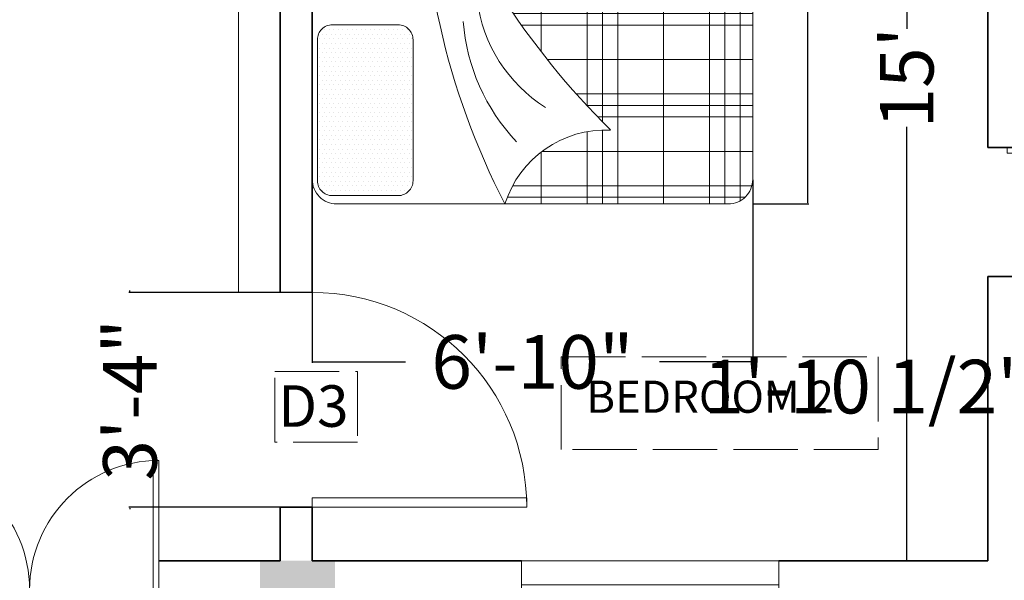
# Model space of a CAD drawing. Units: inches. Extents: x -269 to 4574, y -694 to 313.
# Tile 4 of 19: x 208 to 391, y -360 to -256. Entities that reach past the tile are written whole.
import ezdxf

# ---------------------------------------------------------------- set-up
doc = ezdxf.new("R2010")
doc.units = ezdxf.units.IN
doc.header["$MEASUREMENT"] = 0
doc.linetypes.add('ACAD_ISO02W100', pattern=[15, 12, -3])
for name, color, linetype, lineweight in [('A-ANNO-FRAM', 7, 'ACAD_ISO02W100', 13), ('A-ANNO-IDEN', 6, 'Continuous', 18), ('A-AREA-IDEN', 6, 'Continuous', 20), ('A-COLS', 5, 'Continuous', 35), ('A-FLOR-CASE', 2, 'Continuous', 18), ('A-FURN', 2, 'Continuous', 18), ('DIMENSION', 5, 'Continuous', 18), ('DOORS', 3, 'Continuous', 18), ('WALL', 1, 'Continuous', 35), ('WINDOWS', 2, 'Continuous', 18)]:
    doc.layers.add(name, color=color, linetype=linetype, lineweight=lineweight)
doc.dimstyles.get("Standard").update_dxf_attribs({"dimtxt": 10, "dimasz": 0.18, "dimexe": 0.18, "dimexo": 0.0625, "dimgap": 0.09, "dimtad": 0, "dimdec": 1, "dimzin": 0, "dimdsep": 46, "dimlunit": 3, "dimtxsty": 'Standard', "dimcen": 0.09, "dimclrt": 7, "dimadec": 0, "dimazin": 0, "dimtfac": 1, "dimtdec": 1, "dimtofl": 0, "dimtmove": 0, "dimatfit": 3, "dimfxl": 1, "dimtolj": 1, "dimtzin": 0, "dimarcsym": 0})

# ---------------------------------------------------------------- blocks, each defined once
blk = doc.blocks.new('*U3')
for p, q in [((0, 0), (0, -6)), ((40, 0), (40, -6))]:
    blk.add_line(p, q)
blk.add_lwpolyline([(0, 0), (0, 40), (1.75, 40), (1.75, 0)], close=True)
blk.add_arc((0, 0), 40, 0, 90)
blk = doc.blocks.new('*X12')
at = {"color": 0}
for p, q in [((266.0625, 456.84375), (266.0625, 456.84375)), ((266.25, 456.9375), (266.25, 456.9375)), ((266.25, 456.75), (266.25, 456.75)), ((266.4375, 457.03125), (266.4375, 457.03125)), ((266.4375, 456.84375), (266.4375, 456.84375)), ((266.625, 456.9375), (266.625, 456.9375)), ((266.625, 456.75), (266.625, 456.75)), ((266.8125, 457.03125), (266.8125, 457.03125)), ((266.8125, 456.84375), (266.8125, 456.84375)), ((267, 456.9375), (267, 456.9375)), ((267, 456.75), (267, 456.75)), ((267.1875, 457.03125), (267.1875, 457.03125)), ((267.1875, 456.84375), (267.1875, 456.84375)), ((267.375, 456.9375), (267.375, 456.9375)), ((267.375, 456.75), (267.375, 456.75)), ((267.5625, 457.03125), (267.5625, 457.03125)), ((267.5625, 456.84375), (267.5625, 456.84375)), ((267.75, 456.9375), (267.75, 456.9375)), ((267.75, 456.75), (267.75, 456.75)), ((267.9375, 457.03125), (267.9375, 457.03125)), ((267.9375, 456.84375), (267.9375, 456.84375)), ((268.125, 456.9375), (268.125, 456.9375)), ((268.125, 456.75), (268.125, 456.75)), ((268.3125, 457.03125), (268.3125, 457.03125)), ((268.3125, 456.84375), (268.3125, 456.84375)), ((268.5, 456.9375), (268.5, 456.9375)), ((268.5, 456.75), (268.5, 456.75)), ((268.6875, 457.03125), (268.6875, 457.03125)), ((268.6875, 456.84375), (268.6875, 456.84375)), ((268.875, 456.9375), (268.875, 456.9375)), ((268.875, 456.75), (268.875, 456.75)), ((269.0625, 457.03125), (269.0625, 457.03125)), ((269.0625, 456.84375), (269.0625, 456.84375)), ((269.25, 456.9375), (269.25, 456.9375)), ((269.25, 456.75), (269.25, 456.75)), ((269.4375, 457.03125), (269.4375, 457.03125)), ((269.4375, 456.84375), (269.4375, 456.84375)), ((269.625, 456.9375), (269.625, 456.9375)), ((269.625, 456.75), (269.625, 456.75)), ((269.8125, 457.03125), (269.8125, 457.03125)), ((269.8125, 456.84375), (269.8125, 456.84375)), ((270, 456.9375), (270, 456.9375)), ((270, 456.75), (270, 456.75)), ((270.1875, 457.03125), (270.1875, 457.03125)), ((270.1875, 456.84375), (270.1875, 456.84375)), ((270.375, 456.9375), (270.375, 456.9375)), ((270.375, 456.75), (270.375, 456.75)), ((270.5625, 457.03125), (270.5625, 457.03125)), ((270.5625, 456.84375), (270.5625, 456.84375)), ((270.75, 456.9375), (270.75, 456.9375)), ((270.75, 456.75), (270.75, 456.75)), ((270.9375, 457.03125), (270.9375, 457.03125)), ((270.9375, 456.84375), (270.9375, 456.84375)), ((271.125, 456.9375), (271.125, 456.9375)), ((271.125, 456.75), (271.125, 456.75)), ((271.3125, 457.03125), (271.3125, 457.03125)), ((271.3125, 456.84375), (271.3125, 456.84375)), ((271.5, 456.9375), (271.5, 456.9375)), ((271.5, 456.75), (271.5, 456.75)), ((271.6875, 457.03125), (271.6875, 457.03125)), ((271.6875, 456.84375), (271.6875, 456.84375)), ((271.875, 456.9375), (271.875, 456.9375)), ((271.875, 456.75), (271.875, 456.75)), ((272.0625, 457.03125), (272.0625, 457.03125)), ((272.0625, 456.84375), (272.0625, 456.84375)), ((272.25, 456.9375), (272.25, 456.9375)), ((272.25, 456.75), (272.25, 456.75)), ((272.4375, 456.84375), (272.4375, 456.84375)), ((272.625, 456.75), (272.625, 456.75)), ((265.875, 456.5625), (265.875, 456.5625)), ((265.875, 456.375), (265.875, 456.375)), ((266.0625, 456.65625), (266.0625, 456.65625)), ((266.0625, 456.46875), (266.0625, 456.46875)), ((266.0625, 456.28125), (266.0625, 456.28125)), ((266.25, 456.5625), (266.25, 456.5625)), ((266.25, 456.375), (266.25, 456.375)), ((266.4375, 456.65625), (266.4375, 456.65625)), ((266.4375, 456.46875), (266.4375, 456.46875)), ((266.4375, 456.28125), (266.4375, 456.28125)), ((266.625, 456.5625), (266.625, 456.5625)), ((266.625, 456.375), (266.625, 456.375)), ((266.8125, 456.65625), (266.8125, 456.65625)), ((266.8125, 456.46875), (266.8125, 456.46875)), ((266.8125, 456.28125), (266.8125, 456.28125)), ((267, 456.5625), (267, 456.5625)), ((267, 456.375), (267, 456.375)), ((267.1875, 456.65625), (267.1875, 456.65625)), ((267.1875, 456.46875), (267.1875, 456.46875)), ((267.1875, 456.28125), (267.1875, 456.28125)), ((267.375, 456.5625), (267.375, 456.5625)), ((267.375, 456.375), (267.375, 456.375)), ((267.5625, 456.65625), (267.5625, 456.65625)), ((267.5625, 456.46875), (267.5625, 456.46875)), ((267.5625, 456.28125), (267.5625, 456.28125)), ((267.75, 456.5625), (267.75, 456.5625)), ((267.75, 456.375), (267.75, 456.375)), ((267.9375, 456.65625), (267.9375, 456.65625)), ((267.9375, 456.46875), (267.9375, 456.46875)), ((267.9375, 456.28125), (267.9375, 456.28125)), ((268.125, 456.5625), (268.125, 456.5625)), ((268.125, 456.375), (268.125, 456.375)), ((268.3125, 456.65625), (268.3125, 456.65625)), ((268.3125, 456.46875), (268.3125, 456.46875)), ((268.3125, 456.28125), (268.3125, 456.28125)), ((268.5, 456.5625), (268.5, 456.5625)), ((268.5, 456.375), (268.5, 456.375)), ((268.6875, 456.65625), (268.6875, 456.65625)), ((268.6875, 456.46875), (268.6875, 456.46875)), ((268.6875, 456.28125), (268.6875, 456.28125)), ((268.875, 456.5625), (268.875, 456.5625)), ((268.875, 456.375), (268.875, 456.375)), ((269.0625, 456.65625), (269.0625, 456.65625)), ((269.0625, 456.46875), (269.0625, 456.46875)), ((269.0625, 456.28125), (269.0625, 456.28125)), ((269.25, 456.5625), (269.25, 456.5625)), ((269.25, 456.375), (269.25, 456.375)), ((269.4375, 456.65625), (269.4375, 456.65625)), ((269.4375, 456.46875), (269.4375, 456.46875)), ((269.4375, 456.28125), (269.4375, 456.28125)), ((269.625, 456.5625), (269.625, 456.5625)), ((269.625, 456.375), (269.625, 456.375)), ((269.8125, 456.65625), (269.8125, 456.65625)), ((269.8125, 456.46875), (269.8125, 456.46875)), ((269.8125, 456.28125), (269.8125, 456.28125)), ((270, 456.5625), (270, 456.5625)), ((270, 456.375), (270, 456.375)), ((270.1875, 456.65625), (270.1875, 456.65625)), ((270.1875, 456.46875), (270.1875, 456.46875)), ((270.1875, 456.28125), (270.1875, 456.28125)), ((270.375, 456.5625), (270.375, 456.5625)), ((270.375, 456.375), (270.375, 456.375)), ((270.5625, 456.65625), (270.5625, 456.65625)), ((270.5625, 456.46875), (270.5625, 456.46875)), ((270.5625, 456.28125), (270.5625, 456.28125)), ((270.75, 456.5625), (270.75, 456.5625)), ((270.75, 456.375), (270.75, 456.375)), ((270.9375, 456.65625), (270.9375, 456.65625)), ((270.9375, 456.46875), (270.9375, 456.46875)), ((270.9375, 456.28125), (270.9375, 456.28125)), ((271.125, 456.5625), (271.125, 456.5625)), ((271.125, 456.375), (271.125, 456.375)), ((271.3125, 456.65625), (271.3125, 456.65625)), ((271.3125, 456.46875), (271.3125, 456.46875)), ((271.3125, 456.28125), (271.3125, 456.28125)), ((271.5, 456.5625), (271.5, 456.5625)), ((271.5, 456.375), (271.5, 456.375)), ((271.6875, 456.65625), (271.6875, 456.65625)), ((271.6875, 456.46875), (271.6875, 456.46875)), ((271.6875, 456.28125), (271.6875, 456.28125)), ((271.875, 456.5625), (271.875, 456.5625)), ((271.875, 456.375), (271.875, 456.375)), ((272.0625, 456.65625), (272.0625, 456.65625)), ((272.0625, 456.46875), (272.0625, 456.46875)), ((272.0625, 456.28125), (272.0625, 456.28125)), ((272.25, 456.5625), (272.25, 456.5625)), ((272.25, 456.375), (272.25, 456.375)), ((272.4375, 456.65625), (272.4375, 456.65625)), ((272.4375, 456.46875), (272.4375, 456.46875)), ((272.4375, 456.28125), (272.4375, 456.28125)), ((272.625, 456.5625), (272.625, 456.5625)), ((272.625, 456.375), (272.625, 456.375)), ((272.8125, 456.46875), (272.8125, 456.46875)), ((272.8125, 456.28125), (272.8125, 456.28125)), ((265.875, 456.1875), (265.875, 456.1875)), ((265.875, 456), (265.875, 456)), ((266.0625, 456.09375), (266.0625, 456.09375)), ((266.0625, 455.90625), (266.0625, 455.90625)), ((266.25, 456.1875), (266.25, 456.1875)), ((266.25, 456), (266.25, 456)), ((266.4375, 456.09375), (266.4375, 456.09375)), ((266.4375, 455.90625), (266.4375, 455.90625)), ((266.625, 456.1875), (266.625, 456.1875)), ((266.625, 456), (266.625, 456)), ((266.8125, 456.09375), (266.8125, 456.09375)), ((266.8125, 455.90625), (266.8125, 455.90625)), ((267, 456.1875), (267, 456.1875)), ((267, 456), (267, 456)), ((267.1875, 456.09375), (267.1875, 456.09375)), ((267.1875, 455.90625), (267.1875, 455.90625)), ((267.375, 456.1875), (267.375, 456.1875)), ((267.375, 456), (267.375, 456)), ((267.5625, 456.09375), (267.5625, 456.09375)), ((267.5625, 455.90625), (267.5625, 455.90625)), ((267.75, 456.1875), (267.75, 456.1875)), ((267.75, 456), (267.75, 456)), ((267.9375, 456.09375), (267.9375, 456.09375)), ((267.9375, 455.90625), (267.9375, 455.90625)), ((268.125, 456.1875), (268.125, 456.1875)), ((268.125, 456), (268.125, 456)), ((268.3125, 456.09375), (268.3125, 456.09375)), ((268.3125, 455.90625), (268.3125, 455.90625)), ((268.5, 456.1875), (268.5, 456.1875)), ((268.5, 456), (268.5, 456)), ((268.6875, 456.09375), (268.6875, 456.09375)), ((268.6875, 455.90625), (268.6875, 455.90625)), ((268.875, 456.1875), (268.875, 456.1875)), ((268.875, 456), (268.875, 456)), ((269.0625, 456.09375), (269.0625, 456.09375)), ((269.0625, 455.90625), (269.0625, 455.90625)), ((269.25, 456.1875), (269.25, 456.1875)), ((269.25, 456), (269.25, 456)), ((269.4375, 456.09375), (269.4375, 456.09375)), ((269.4375, 455.90625), (269.4375, 455.90625)), ((269.625, 456.1875), (269.625, 456.1875)), ((269.625, 456), (269.625, 456)), ((269.8125, 456.09375), (269.8125, 456.09375)), ((269.8125, 455.90625), (269.8125, 455.90625)), ((270, 456.1875), (270, 456.1875)), ((270, 456), (270, 456)), ((270.1875, 456.09375), (270.1875, 456.09375)), ((270.1875, 455.90625), (270.1875, 455.90625)), ((270.375, 456.1875), (270.375, 456.1875)), ((270.375, 456), (270.375, 456)), ((270.5625, 456.09375), (270.5625, 456.09375)), ((270.5625, 455.90625), (270.5625, 455.90625)), ((270.75, 456.1875), (270.75, 456.1875)), ((270.75, 456), (270.75, 456)), ((270.9375, 456.09375), (270.9375, 456.09375)), ((270.9375, 455.90625), (270.9375, 455.90625)), ((271.125, 456.1875), (271.125, 456.1875)), ((271.125, 456), (271.125, 456)), ((271.3125, 456.09375), (271.3125, 456.09375)), ((271.3125, 455.90625), (271.3125, 455.90625)), ((271.5, 456.1875), (271.5, 456.1875)), ((271.5, 456), (271.5, 456)), ((271.6875, 456.09375), (271.6875, 456.09375)), ((271.6875, 455.90625), (271.6875, 455.90625)), ((271.875, 456.1875), (271.875, 456.1875)), ((271.875, 456), (271.875, 456)), ((272.0625, 456.09375), (272.0625, 456.09375)), ((272.0625, 455.90625), (272.0625, 455.90625)), ((272.25, 456.1875), (272.25, 456.1875)), ((272.25, 456), (272.25, 456)), ((272.4375, 456.09375), (272.4375, 456.09375)), ((272.4375, 455.90625), (272.4375, 455.90625)), ((272.625, 456.1875), (272.625, 456.1875)), ((272.625, 456), (272.625, 456)), ((272.8125, 456.09375), (272.8125, 456.09375)), ((272.8125, 455.90625), (272.8125, 455.90625)), ((265.875, 455.8125), (265.875, 455.8125)), ((265.875, 455.625), (265.875, 455.625)), ((266.0625, 455.71875), (266.0625, 455.71875)), ((266.0625, 455.53125), (266.0625, 455.53125)), ((266.25, 455.8125), (266.25, 455.8125)), ((266.25, 455.625), (266.25, 455.625)), ((266.4375, 455.71875), (266.4375, 455.71875)), ((266.4375, 455.53125), (266.4375, 455.53125)), ((266.625, 455.8125), (266.625, 455.8125)), ((266.625, 455.625), (266.625, 455.625)), ((266.8125, 455.71875), (266.8125, 455.71875)), ((266.8125, 455.53125), (266.8125, 455.53125)), ((267, 455.8125), (267, 455.8125)), ((267, 455.625), (267, 455.625)), ((267.1875, 455.71875), (267.1875, 455.71875)), ((267.1875, 455.53125), (267.1875, 455.53125)), ((267.375, 455.8125), (267.375, 455.8125)), ((267.375, 455.625), (267.375, 455.625)), ((267.5625, 455.71875), (267.5625, 455.71875)), ((267.5625, 455.53125), (267.5625, 455.53125)), ((267.75, 455.8125), (267.75, 455.8125)), ((267.75, 455.625), (267.75, 455.625)), ((267.9375, 455.71875), (267.9375, 455.71875)), ((267.9375, 455.53125), (267.9375, 455.53125)), ((268.125, 455.8125), (268.125, 455.8125)), ((268.125, 455.625), (268.125, 455.625)), ((268.3125, 455.71875), (268.3125, 455.71875)), ((268.3125, 455.53125), (268.3125, 455.53125)), ((268.5, 455.8125), (268.5, 455.8125)), ((268.5, 455.625), (268.5, 455.625)), ((268.6875, 455.71875), (268.6875, 455.71875)), ((268.6875, 455.53125), (268.6875, 455.53125)), ((268.875, 455.8125), (268.875, 455.8125)), ((268.875, 455.625), (268.875, 455.625)), ((269.0625, 455.71875), (269.0625, 455.71875)), ((269.0625, 455.53125), (269.0625, 455.53125)), ((269.25, 455.8125), (269.25, 455.8125)), ((269.25, 455.625), (269.25, 455.625)), ((269.4375, 455.71875), (269.4375, 455.71875)), ((269.4375, 455.53125), (269.4375, 455.53125)), ((269.625, 455.8125), (269.625, 455.8125)), ((269.625, 455.625), (269.625, 455.625)), ((269.8125, 455.71875), (269.8125, 455.71875)), ((269.8125, 455.53125), (269.8125, 455.53125)), ((270, 455.8125), (270, 455.8125)), ((270, 455.625), (270, 455.625)), ((270.1875, 455.71875), (270.1875, 455.71875)), ((270.1875, 455.53125), (270.1875, 455.53125)), ((270.375, 455.8125), (270.375, 455.8125)), ((270.375, 455.625), (270.375, 455.625)), ((270.5625, 455.71875), (270.5625, 455.71875)), ((270.5625, 455.53125), (270.5625, 455.53125)), ((270.75, 455.8125), (270.75, 455.8125)), ((270.75, 455.625), (270.75, 455.625)), ((270.9375, 455.71875), (270.9375, 455.71875)), ((270.9375, 455.53125), (270.9375, 455.53125)), ((271.125, 455.8125), (271.125, 455.8125)), ((271.125, 455.625), (271.125, 455.625)), ((271.3125, 455.71875), (271.3125, 455.71875)), ((271.3125, 455.53125), (271.3125, 455.53125)), ((271.5, 455.8125), (271.5, 455.8125)), ((271.5, 455.625), (271.5, 455.625)), ((271.6875, 455.71875), (271.6875, 455.71875)), ((271.6875, 455.53125), (271.6875, 455.53125)), ((271.875, 455.8125), (271.875, 455.8125)), ((271.875, 455.625), (271.875, 455.625)), ((272.0625, 455.71875), (272.0625, 455.71875)), ((272.0625, 455.53125), (272.0625, 455.53125)), ((272.25, 455.8125), (272.25, 455.8125)), ((272.25, 455.625), (272.25, 455.625)), ((272.4375, 455.71875), (272.4375, 455.71875)), ((272.4375, 455.53125), (272.4375, 455.53125)), ((272.625, 455.8125), (272.625, 455.8125)), ((272.625, 455.625), (272.625, 455.625)), ((272.8125, 455.71875), (272.8125, 455.71875)), ((272.8125, 455.53125), (272.8125, 455.53125)), ((265.875, 455.4375), (265.875, 455.4375)), ((265.875, 455.25), (265.875, 455.25)), ((266.0625, 455.34375), (266.0625, 455.34375)), ((266.0625, 455.15625), (266.0625, 455.15625)), ((266.25, 455.4375), (266.25, 455.4375)), ((266.25, 455.25), (266.25, 455.25)), ((266.4375, 455.34375), (266.4375, 455.34375)), ((266.4375, 455.15625), (266.4375, 455.15625)), ((266.625, 455.4375), (266.625, 455.4375)), ((266.625, 455.25), (266.625, 455.25)), ((266.8125, 455.34375), (266.8125, 455.34375)), ((266.8125, 455.15625), (266.8125, 455.15625)), ((267, 455.4375), (267, 455.4375)), ((267, 455.25), (267, 455.25)), ((267.1875, 455.34375), (267.1875, 455.34375)), ((267.1875, 455.15625), (267.1875, 455.15625)), ((267.375, 455.4375), (267.375, 455.4375)), ((267.375, 455.25), (267.375, 455.25)), ((267.5625, 455.34375), (267.5625, 455.34375)), ((267.5625, 455.15625), (267.5625, 455.15625)), ((267.75, 455.4375), (267.75, 455.4375)), ((267.75, 455.25), (267.75, 455.25)), ((267.9375, 455.34375), (267.9375, 455.34375)), ((267.9375, 455.15625), (267.9375, 455.15625)), ((268.125, 455.4375), (268.125, 455.4375)), ((268.125, 455.25), (268.125, 455.25)), ((268.3125, 455.34375), (268.3125, 455.34375)), ((268.3125, 455.15625), (268.3125, 455.15625)), ((268.5, 455.4375), (268.5, 455.4375)), ((268.5, 455.25), (268.5, 455.25)), ((268.6875, 455.34375), (268.6875, 455.34375)), ((268.6875, 455.15625), (268.6875, 455.15625)), ((268.875, 455.4375), (268.875, 455.4375)), ((268.875, 455.25), (268.875, 455.25)), ((269.0625, 455.34375), (269.0625, 455.34375)), ((269.0625, 455.15625), (269.0625, 455.15625)), ((269.25, 455.4375), (269.25, 455.4375)), ((269.25, 455.25), (269.25, 455.25)), ((269.4375, 455.34375), (269.4375, 455.34375)), ((269.4375, 455.15625), (269.4375, 455.15625)), ((269.625, 455.4375), (269.625, 455.4375)), ((269.625, 455.25), (269.625, 455.25)), ((269.8125, 455.34375), (269.8125, 455.34375)), ((269.8125, 455.15625), (269.8125, 455.15625)), ((270, 455.4375), (270, 455.4375)), ((270, 455.25), (270, 455.25)), ((270.1875, 455.34375), (270.1875, 455.34375)), ((270.1875, 455.15625), (270.1875, 455.15625)), ((270.375, 455.4375), (270.375, 455.4375)), ((270.375, 455.25), (270.375, 455.25)), ((270.5625, 455.34375), (270.5625, 455.34375)), ((270.5625, 455.15625), (270.5625, 455.15625)), ((270.75, 455.4375), (270.75, 455.4375)), ((270.75, 455.25), (270.75, 455.25)), ((270.9375, 455.34375), (270.9375, 455.34375)), ((270.9375, 455.15625), (270.9375, 455.15625)), ((271.125, 455.4375), (271.125, 455.4375)), ((271.125, 455.25), (271.125, 455.25)), ((271.3125, 455.34375), (271.3125, 455.34375)), ((271.3125, 455.15625), (271.3125, 455.15625)), ((271.5, 455.4375), (271.5, 455.4375)), ((271.5, 455.25), (271.5, 455.25)), ((271.6875, 455.34375), (271.6875, 455.34375)), ((271.6875, 455.15625), (271.6875, 455.15625)), ((271.875, 455.4375), (271.875, 455.4375)), ((271.875, 455.25), (271.875, 455.25)), ((272.0625, 455.34375), (272.0625, 455.34375)), ((272.0625, 455.15625), (272.0625, 455.15625)), ((272.25, 455.4375), (272.25, 455.4375)), ((272.25, 455.25), (272.25, 455.25)), ((272.4375, 455.34375), (272.4375, 455.34375)), ((272.4375, 455.15625), (272.4375, 455.15625)), ((272.625, 455.4375), (272.625, 455.4375)), ((272.625, 455.25), (272.625, 455.25)), ((272.8125, 455.34375), (272.8125, 455.34375)), ((272.8125, 455.15625), (272.8125, 455.15625)), ((265.875, 455.0625), (265.875, 455.0625)), ((265.875, 454.875), (265.875, 454.875)), ((265.875, 454.6875), (265.875, 454.6875)), ((266.0625, 454.96875), (266.0625, 454.96875)), ((266.0625, 454.78125), (266.0625, 454.78125)), ((266.25, 455.0625), (266.25, 455.0625)), ((266.25, 454.875), (266.25, 454.875)), ((266.25, 454.6875), (266.25, 454.6875)), ((266.4375, 454.96875), (266.4375, 454.96875)), ((266.4375, 454.78125), (266.4375, 454.78125)), ((266.625, 455.0625), (266.625, 455.0625)), ((266.625, 454.875), (266.625, 454.875)), ((266.625, 454.6875), (266.625, 454.6875)), ((266.8125, 454.96875), (266.8125, 454.96875)), ((266.8125, 454.78125), (266.8125, 454.78125)), ((267, 455.0625), (267, 455.0625)), ((267, 454.875), (267, 454.875)), ((267, 454.6875), (267, 454.6875)), ((267.1875, 454.96875), (267.1875, 454.96875)), ((267.1875, 454.78125), (267.1875, 454.78125)), ((267.375, 455.0625), (267.375, 455.0625)), ((267.375, 454.875), (267.375, 454.875)), ((267.375, 454.6875), (267.375, 454.6875)), ((267.5625, 454.96875), (267.5625, 454.96875)), ((267.5625, 454.78125), (267.5625, 454.78125)), ((267.75, 455.0625), (267.75, 455.0625)), ((267.75, 454.875), (267.75, 454.875)), ((267.75, 454.6875), (267.75, 454.6875)), ((267.9375, 454.96875), (267.9375, 454.96875)), ((267.9375, 454.78125), (267.9375, 454.78125)), ((268.125, 455.0625), (268.125, 455.0625)), ((268.125, 454.875), (268.125, 454.875)), ((268.125, 454.6875), (268.125, 454.6875)), ((268.3125, 454.96875), (268.3125, 454.96875)), ((268.3125, 454.78125), (268.3125, 454.78125)), ((268.5, 455.0625), (268.5, 455.0625)), ((268.5, 454.875), (268.5, 454.875)), ((268.5, 454.6875), (268.5, 454.6875)), ((268.6875, 454.96875), (268.6875, 454.96875)), ((268.6875, 454.78125), (268.6875, 454.78125)), ((268.875, 455.0625), (268.875, 455.0625)), ((268.875, 454.875), (268.875, 454.875)), ((268.875, 454.6875), (268.875, 454.6875)), ((269.0625, 454.96875), (269.0625, 454.96875)), ((269.0625, 454.78125), (269.0625, 454.78125)), ((269.25, 455.0625), (269.25, 455.0625)), ((269.25, 454.875), (269.25, 454.875)), ((269.25, 454.6875), (269.25, 454.6875)), ((269.4375, 454.96875), (269.4375, 454.96875)), ((269.4375, 454.78125), (269.4375, 454.78125)), ((269.625, 455.0625), (269.625, 455.0625)), ((269.625, 454.875), (269.625, 454.875)), ((269.625, 454.6875), (269.625, 454.6875)), ((269.8125, 454.96875), (269.8125, 454.96875)), ((269.8125, 454.78125), (269.8125, 454.78125)), ((270, 455.0625), (270, 455.0625)), ((270, 454.875), (270, 454.875)), ((270, 454.6875), (270, 454.6875)), ((270.1875, 454.96875), (270.1875, 454.96875)), ((270.1875, 454.78125), (270.1875, 454.78125)), ((270.375, 455.0625), (270.375, 455.0625)), ((270.375, 454.875), (270.375, 454.875)), ((270.375, 454.6875), (270.375, 454.6875)), ((270.5625, 454.96875), (270.5625, 454.96875)), ((270.5625, 454.78125), (270.5625, 454.78125)), ((270.75, 455.0625), (270.75, 455.0625)), ((270.75, 454.875), (270.75, 454.875)), ((270.75, 454.6875), (270.75, 454.6875)), ((270.9375, 454.96875), (270.9375, 454.96875)), ((270.9375, 454.78125), (270.9375, 454.78125)), ((271.125, 455.0625), (271.125, 455.0625)), ((271.125, 454.875), (271.125, 454.875)), ((271.125, 454.6875), (271.125, 454.6875)), ((271.3125, 454.96875), (271.3125, 454.96875)), ((271.3125, 454.78125), (271.3125, 454.78125)), ((271.5, 455.0625), (271.5, 455.0625)), ((271.5, 454.875), (271.5, 454.875)), ((271.5, 454.6875), (271.5, 454.6875)), ((271.6875, 454.96875), (271.6875, 454.96875)), ((271.6875, 454.78125), (271.6875, 454.78125)), ((271.875, 455.0625), (271.875, 455.0625)), ((271.875, 454.875), (271.875, 454.875)), ((271.875, 454.6875), (271.875, 454.6875)), ((272.0625, 454.96875), (272.0625, 454.96875)), ((272.0625, 454.78125), (272.0625, 454.78125)), ((272.25, 455.0625), (272.25, 455.0625)), ((272.25, 454.875), (272.25, 454.875)), ((272.25, 454.6875), (272.25, 454.6875)), ((272.4375, 454.96875), (272.4375, 454.96875)), ((272.4375, 454.78125), (272.4375, 454.78125)), ((272.625, 455.0625), (272.625, 455.0625)), ((272.625, 454.875), (272.625, 454.875)), ((272.625, 454.6875), (272.625, 454.6875)), ((272.8125, 454.96875), (272.8125, 454.96875)), ((272.8125, 454.78125), (272.8125, 454.78125)), ((265.875, 454.5), (265.875, 454.5)), ((265.875, 454.3125), (265.875, 454.3125)), ((266.0625, 454.59375), (266.0625, 454.59375)), ((266.0625, 454.40625), (266.0625, 454.40625)), ((266.25, 454.5), (266.25, 454.5)), ((266.25, 454.3125), (266.25, 454.3125)), ((266.4375, 454.59375), (266.4375, 454.59375)), ((266.4375, 454.40625), (266.4375, 454.40625)), ((266.625, 454.5), (266.625, 454.5)), ((266.625, 454.3125), (266.625, 454.3125)), ((266.8125, 454.59375), (266.8125, 454.59375)), ((266.8125, 454.40625), (266.8125, 454.40625)), ((267, 454.5), (267, 454.5)), ((267, 454.3125), (267, 454.3125)), ((267.1875, 454.59375), (267.1875, 454.59375)), ((267.1875, 454.40625), (267.1875, 454.40625)), ((267.375, 454.5), (267.375, 454.5)), ((267.375, 454.3125), (267.375, 454.3125)), ((267.5625, 454.59375), (267.5625, 454.59375)), ((267.5625, 454.40625), (267.5625, 454.40625)), ((267.75, 454.5), (267.75, 454.5)), ((267.75, 454.3125), (267.75, 454.3125)), ((267.9375, 454.59375), (267.9375, 454.59375)), ((267.9375, 454.40625), (267.9375, 454.40625)), ((268.125, 454.5), (268.125, 454.5)), ((268.125, 454.3125), (268.125, 454.3125)), ((268.3125, 454.59375), (268.3125, 454.59375)), ((268.3125, 454.40625), (268.3125, 454.40625)), ((268.5, 454.5), (268.5, 454.5)), ((268.5, 454.3125), (268.5, 454.3125)), ((268.6875, 454.59375), (268.6875, 454.59375)), ((268.6875, 454.40625), (268.6875, 454.40625)), ((268.875, 454.5), (268.875, 454.5)), ((268.875, 454.3125), (268.875, 454.3125)), ((269.0625, 454.59375), (269.0625, 454.59375)), ((269.0625, 454.40625), (269.0625, 454.40625)), ((269.25, 454.5), (269.25, 454.5)), ((269.25, 454.3125), (269.25, 454.3125)), ((269.4375, 454.59375), (269.4375, 454.59375)), ((269.4375, 454.40625), (269.4375, 454.40625)), ((269.625, 454.5), (269.625, 454.5)), ((269.625, 454.3125), (269.625, 454.3125)), ((269.8125, 454.59375), (269.8125, 454.59375)), ((269.8125, 454.40625), (269.8125, 454.40625)), ((270, 454.5), (270, 454.5)), ((270, 454.3125), (270, 454.3125)), ((270.1875, 454.59375), (270.1875, 454.59375)), ((270.1875, 454.40625), (270.1875, 454.40625)), ((270.375, 454.5), (270.375, 454.5)), ((270.375, 454.3125), (270.375, 454.3125)), ((270.5625, 454.59375), (270.5625, 454.59375)), ((270.5625, 454.40625), (270.5625, 454.40625)), ((270.75, 454.5), (270.75, 454.5)), ((270.75, 454.3125), (270.75, 454.3125)), ((270.9375, 454.59375), (270.9375, 454.59375)), ((270.9375, 454.40625), (270.9375, 454.40625)), ((271.125, 454.5), (271.125, 454.5)), ((271.125, 454.3125), (271.125, 454.3125)), ((271.3125, 454.59375), (271.3125, 454.59375)), ((271.3125, 454.40625), (271.3125, 454.40625)), ((271.5, 454.5), (271.5, 454.5)), ((271.5, 454.3125), (271.5, 454.3125)), ((271.6875, 454.59375), (271.6875, 454.59375)), ((271.6875, 454.40625), (271.6875, 454.40625)), ((271.875, 454.5), (271.875, 454.5)), ((271.875, 454.3125), (271.875, 454.3125)), ((272.0625, 454.59375), (272.0625, 454.59375)), ((272.0625, 454.40625), (272.0625, 454.40625)), ((272.25, 454.5), (272.25, 454.5)), ((272.25, 454.3125), (272.25, 454.3125)), ((272.4375, 454.59375), (272.4375, 454.59375)), ((272.4375, 454.40625), (272.4375, 454.40625)), ((272.625, 454.5), (272.625, 454.5)), ((272.625, 454.3125), (272.625, 454.3125)), ((272.8125, 454.59375), (272.8125, 454.59375)), ((272.8125, 454.40625), (272.8125, 454.40625)), ((265.875, 454.125), (265.875, 454.125)), ((265.875, 453.9375), (265.875, 453.9375)), ((266.0625, 454.21875), (266.0625, 454.21875)), ((266.0625, 454.03125), (266.0625, 454.03125)), ((266.25, 454.125), (266.25, 454.125)), ((266.25, 453.9375), (266.25, 453.9375)), ((266.4375, 454.21875), (266.4375, 454.21875)), ((266.4375, 454.03125), (266.4375, 454.03125)), ((266.625, 454.125), (266.625, 454.125)), ((266.625, 453.9375), (266.625, 453.9375)), ((266.8125, 454.21875), (266.8125, 454.21875)), ((266.8125, 454.03125), (266.8125, 454.03125)), ((267, 454.125), (267, 454.125)), ((267, 453.9375), (267, 453.9375)), ((267.1875, 454.21875), (267.1875, 454.21875)), ((267.1875, 454.03125), (267.1875, 454.03125)), ((267.375, 454.125), (267.375, 454.125)), ((267.375, 453.9375), (267.375, 453.9375)), ((267.5625, 454.21875), (267.5625, 454.21875)), ((267.5625, 454.03125), (267.5625, 454.03125)), ((267.75, 454.125), (267.75, 454.125)), ((267.75, 453.9375), (267.75, 453.9375)), ((267.9375, 454.21875), (267.9375, 454.21875)), ((267.9375, 454.03125), (267.9375, 454.03125)), ((268.125, 454.125), (268.125, 454.125)), ((268.125, 453.9375), (268.125, 453.9375)), ((268.3125, 454.21875), (268.3125, 454.21875)), ((268.3125, 454.03125), (268.3125, 454.03125)), ((268.5, 454.125), (268.5, 454.125)), ((268.5, 453.9375), (268.5, 453.9375)), ((268.6875, 454.21875), (268.6875, 454.21875)), ((268.6875, 454.03125), (268.6875, 454.03125)), ((268.875, 454.125), (268.875, 454.125)), ((268.875, 453.9375), (268.875, 453.9375)), ((269.0625, 454.21875), (269.0625, 454.21875)), ((269.0625, 454.03125), (269.0625, 454.03125)), ((269.25, 454.125), (269.25, 454.125)), ((269.25, 453.9375), (269.25, 453.9375)), ((269.4375, 454.21875), (269.4375, 454.21875)), ((269.4375, 454.03125), (269.4375, 454.03125)), ((269.625, 454.125), (269.625, 454.125)), ((269.625, 453.9375), (269.625, 453.9375)), ((269.8125, 454.21875), (269.8125, 454.21875)), ((269.8125, 454.03125), (269.8125, 454.03125)), ((270, 454.125), (270, 454.125)), ((270, 453.9375), (270, 453.9375)), ((270.1875, 454.21875), (270.1875, 454.21875)), ((270.1875, 454.03125), (270.1875, 454.03125)), ((270.375, 454.125), (270.375, 454.125)), ((270.375, 453.9375), (270.375, 453.9375)), ((270.5625, 454.21875), (270.5625, 454.21875)), ((270.5625, 454.03125), (270.5625, 454.03125)), ((270.75, 454.125), (270.75, 454.125)), ((270.75, 453.9375), (270.75, 453.9375)), ((270.9375, 454.21875), (270.9375, 454.21875)), ((270.9375, 454.03125), (270.9375, 454.03125)), ((271.125, 454.125), (271.125, 454.125)), ((271.125, 453.9375), (271.125, 453.9375)), ((271.3125, 454.21875), (271.3125, 454.21875)), ((271.3125, 454.03125), (271.3125, 454.03125)), ((271.5, 454.125), (271.5, 454.125)), ((271.5, 453.9375), (271.5, 453.9375)), ((271.6875, 454.21875), (271.6875, 454.21875)), ((271.6875, 454.03125), (271.6875, 454.03125)), ((271.875, 454.125), (271.875, 454.125)), ((271.875, 453.9375), (271.875, 453.9375)), ((272.0625, 454.21875), (272.0625, 454.21875)), ((272.0625, 454.03125), (272.0625, 454.03125)), ((272.25, 454.125), (272.25, 454.125)), ((272.25, 453.9375), (272.25, 453.9375)), ((272.4375, 454.21875), (272.4375, 454.21875)), ((272.4375, 454.03125), (272.4375, 454.03125)), ((272.625, 454.125), (272.625, 454.125)), ((272.625, 453.9375), (272.625, 453.9375)), ((272.8125, 454.21875), (272.8125, 454.21875)), ((272.8125, 454.03125), (272.8125, 454.03125)), ((265.875, 453.75), (265.875, 453.75)), ((266.0625, 453.84375), (266.0625, 453.84375)), ((266.0625, 453.65625), (266.0625, 453.65625)), ((266.0625, 453.46875), (266.0625, 453.46875)), ((266.25, 453.75), (266.25, 453.75)), ((266.25, 453.5625), (266.25, 453.5625)), ((266.4375, 453.84375), (266.4375, 453.84375)), ((266.4375, 453.65625), (266.4375, 453.65625)), ((266.4375, 453.46875), (266.4375, 453.46875)), ((266.625, 453.75), (266.625, 453.75)), ((266.625, 453.5625), (266.625, 453.5625)), ((266.8125, 453.84375), (266.8125, 453.84375)), ((266.8125, 453.65625), (266.8125, 453.65625)), ((266.8125, 453.46875), (266.8125, 453.46875)), ((267, 453.75), (267, 453.75)), ((267, 453.5625), (267, 453.5625)), ((267.1875, 453.84375), (267.1875, 453.84375)), ((267.1875, 453.65625), (267.1875, 453.65625)), ((267.1875, 453.46875), (267.1875, 453.46875)), ((267.375, 453.75), (267.375, 453.75)), ((267.375, 453.5625), (267.375, 453.5625)), ((267.5625, 453.84375), (267.5625, 453.84375)), ((267.5625, 453.65625), (267.5625, 453.65625)), ((267.5625, 453.46875), (267.5625, 453.46875)), ((267.75, 453.75), (267.75, 453.75)), ((267.75, 453.5625), (267.75, 453.5625)), ((267.9375, 453.84375), (267.9375, 453.84375)), ((267.9375, 453.65625), (267.9375, 453.65625)), ((267.9375, 453.46875), (267.9375, 453.46875)), ((268.125, 453.75), (268.125, 453.75)), ((268.125, 453.5625), (268.125, 453.5625)), ((268.3125, 453.84375), (268.3125, 453.84375)), ((268.3125, 453.65625), (268.3125, 453.65625)), ((268.3125, 453.46875), (268.3125, 453.46875)), ((268.5, 453.75), (268.5, 453.75)), ((268.5, 453.5625), (268.5, 453.5625)), ((268.6875, 453.84375), (268.6875, 453.84375)), ((268.6875, 453.65625), (268.6875, 453.65625)), ((268.6875, 453.46875), (268.6875, 453.46875)), ((268.875, 453.75), (268.875, 453.75)), ((268.875, 453.5625), (268.875, 453.5625)), ((269.0625, 453.84375), (269.0625, 453.84375)), ((269.0625, 453.65625), (269.0625, 453.65625)), ((269.0625, 453.46875), (269.0625, 453.46875)), ((269.25, 453.75), (269.25, 453.75)), ((269.25, 453.5625), (269.25, 453.5625)), ((269.4375, 453.84375), (269.4375, 453.84375)), ((269.4375, 453.65625), (269.4375, 453.65625)), ((269.4375, 453.46875), (269.4375, 453.46875)), ((269.625, 453.75), (269.625, 453.75)), ((269.625, 453.5625), (269.625, 453.5625)), ((269.8125, 453.84375), (269.8125, 453.84375)), ((269.8125, 453.65625), (269.8125, 453.65625)), ((269.8125, 453.46875), (269.8125, 453.46875)), ((270, 453.75), (270, 453.75)), ((270, 453.5625), (270, 453.5625)), ((270.1875, 453.84375), (270.1875, 453.84375)), ((270.1875, 453.65625), (270.1875, 453.65625)), ((270.1875, 453.46875), (270.1875, 453.46875)), ((270.375, 453.75), (270.375, 453.75)), ((270.375, 453.5625), (270.375, 453.5625)), ((270.5625, 453.84375), (270.5625, 453.84375)), ((270.5625, 453.65625), (270.5625, 453.65625)), ((270.5625, 453.46875), (270.5625, 453.46875)), ((270.75, 453.75), (270.75, 453.75)), ((270.75, 453.5625), (270.75, 453.5625)), ((270.9375, 453.84375), (270.9375, 453.84375)), ((270.9375, 453.65625), (270.9375, 453.65625)), ((270.9375, 453.46875), (270.9375, 453.46875)), ((271.125, 453.75), (271.125, 453.75)), ((271.125, 453.5625), (271.125, 453.5625)), ((271.3125, 453.84375), (271.3125, 453.84375)), ((271.3125, 453.65625), (271.3125, 453.65625)), ((271.3125, 453.46875), (271.3125, 453.46875)), ((271.5, 453.75), (271.5, 453.75)), ((271.5, 453.5625), (271.5, 453.5625)), ((271.6875, 453.84375), (271.6875, 453.84375)), ((271.6875, 453.65625), (271.6875, 453.65625)), ((271.6875, 453.46875), (271.6875, 453.46875)), ((271.875, 453.75), (271.875, 453.75)), ((271.875, 453.5625), (271.875, 453.5625)), ((272.0625, 453.84375), (272.0625, 453.84375)), ((272.0625, 453.65625), (272.0625, 453.65625)), ((272.0625, 453.46875), (272.0625, 453.46875)), ((272.25, 453.75), (272.25, 453.75)), ((272.25, 453.5625), (272.25, 453.5625)), ((272.4375, 453.84375), (272.4375, 453.84375)), ((272.4375, 453.65625), (272.4375, 453.65625)), ((272.4375, 453.46875), (272.4375, 453.46875)), ((272.625, 453.75), (272.625, 453.75)), ((272.625, 453.5625), (272.625, 453.5625)), ((272.8125, 453.84375), (272.8125, 453.84375)), ((272.8125, 453.65625), (272.8125, 453.65625)), ((266.0625, 453.28125), (266.0625, 453.28125)), ((266.25, 453.375), (266.25, 453.375)), ((266.25, 453.1875), (266.25, 453.1875)), ((266.4375, 453.28125), (266.4375, 453.28125)), ((266.625, 453.375), (266.625, 453.375)), ((266.625, 453.1875), (266.625, 453.1875)), ((266.8125, 453.28125), (266.8125, 453.28125)), ((267, 453.375), (267, 453.375)), ((267, 453.1875), (267, 453.1875)), ((267.1875, 453.28125), (267.1875, 453.28125)), ((267.375, 453.375), (267.375, 453.375)), ((267.375, 453.1875), (267.375, 453.1875)), ((267.5625, 453.28125), (267.5625, 453.28125)), ((267.75, 453.375), (267.75, 453.375)), ((267.75, 453.1875), (267.75, 453.1875)), ((267.9375, 453.28125), (267.9375, 453.28125)), ((268.125, 453.375), (268.125, 453.375)), ((268.125, 453.1875), (268.125, 453.1875)), ((268.3125, 453.28125), (268.3125, 453.28125)), ((268.5, 453.375), (268.5, 453.375)), ((268.5, 453.1875), (268.5, 453.1875)), ((268.6875, 453.28125), (268.6875, 453.28125)), ((268.875, 453.375), (268.875, 453.375)), ((268.875, 453.1875), (268.875, 453.1875)), ((269.0625, 453.28125), (269.0625, 453.28125)), ((269.25, 453.375), (269.25, 453.375)), ((269.25, 453.1875), (269.25, 453.1875)), ((269.4375, 453.28125), (269.4375, 453.28125)), ((269.625, 453.375), (269.625, 453.375)), ((269.625, 453.1875), (269.625, 453.1875)), ((269.8125, 453.28125), (269.8125, 453.28125)), ((270, 453.375), (270, 453.375)), ((270, 453.1875), (270, 453.1875)), ((270.1875, 453.28125), (270.1875, 453.28125)), ((270.375, 453.375), (270.375, 453.375)), ((270.375, 453.1875), (270.375, 453.1875)), ((270.5625, 453.28125), (270.5625, 453.28125)), ((270.75, 453.375), (270.75, 453.375)), ((270.75, 453.1875), (270.75, 453.1875)), ((270.9375, 453.28125), (270.9375, 453.28125)), ((271.125, 453.375), (271.125, 453.375)), ((271.125, 453.1875), (271.125, 453.1875)), ((271.3125, 453.28125), (271.3125, 453.28125)), ((271.5, 453.375), (271.5, 453.375)), ((271.5, 453.1875), (271.5, 453.1875)), ((271.6875, 453.28125), (271.6875, 453.28125)), ((271.875, 453.375), (271.875, 453.375)), ((271.875, 453.1875), (271.875, 453.1875)), ((272.0625, 453.28125), (272.0625, 453.28125)), ((272.25, 453.375), (272.25, 453.375)), ((272.25, 453.1875), (272.25, 453.1875)), ((272.4375, 453.28125), (272.4375, 453.28125)), ((272.625, 453.375), (272.625, 453.375))]:
    blk.add_line(p, q, dxfattribs=at)
blk = doc.blocks.new('*D22')
at = {"layer": 'Defpoints', "color": 0, "lineweight": 0, "transparency": 16777216}
for p in [(372.99, -176.73), (388.14, -176.73), (388.14, -356.73)]:
    blk.add_point(p, dxfattribs=at)
at = {"layer": 'DIMENSION', "color": 0, "lineweight": -2, "transparency": 16777216}
for p, q in [((388.07, -176.73), (372.81, -176.73)), ((372.99, -176.91), (372.99, -257.59)), ((372.99, -356.55), (372.99, -275.87)), ((388.07, -356.73), (372.81, -356.73))]:
    blk.add_line(p, q, dxfattribs=at)
at = {"layer": 'DIMENSION', "color": 0, "lineweight": 0, "transparency": 16777216}
for points in [[(372.96, -176.91), (373.02, -176.91), (372.99, -176.73)], [(372.96, -356.55), (373.02, -356.55), (372.99, -356.73)]]:
    blk.add_solid(points, dxfattribs=at)
at = {"layer": 'DIMENSION', "color": 0, "transparency": 16777216, "insert": (372.99, -266.73), "char_height": 10, "attachment_point": 5, "rotation": 90}
blk.add_mtext("\\A1;15'", dxfattribs=at)
blk = doc.blocks.new('GLAZ-48IN')
blk.add_line((4.5, 0), (4.5, 48))
blk.add_lwpolyline([(0, 48), (9, 48), (9, 0), (0, 0)], close=True)
blk = doc.blocks.new('*X10')
at = {"color": 0}
for p, q in [((276.598, 451.25), (280.51, 451.25)), ((275.455, 450.625), (280.51, 450.625)), ((274.411, 450), (280.51, 450)), ((265.51, 448.125), (267.634, 448.125)), ((271.723, 448.125), (280.51, 448.125)), ((265.51, 446.25), (268.465, 446.25)), ((269.519, 446.25), (280.51, 446.25)), ((265.51, 445.625), (268.531, 445.625)), ((268.866, 445.625), (280.51, 445.625)), ((265.51, 445), (280.51, 445)), ((265.51, 443.125), (280.51, 443.125)), ((265.51, 441.25), (280.51, 441.25)), ((265.51, 440.625), (280.51, 440.625)), ((265.634, 440), (280.386, 440))]:
    blk.add_line(p, q, dxfattribs=at)
blk = doc.blocks.new('*X11')
at = {"color": 0}
for p, q in [((280.312, 439.886), (280.312, 452.896)), ((278.906, 439.482), (278.906, 452.338)), ((277.031, 439.482), (277.031, 451.471)), ((277.5, 439.482), (277.5, 451.702)), ((276.562, 439.482), (276.562, 451.231)), ((275.156, 439.482), (275.156, 450.451)), ((265.781, 439.797), (265.781, 449.511)), ((273.75, 439.482), (273.75, 449.576)), ((266.25, 439.517), (266.25, 449.296)), ((273.281, 439.482), (273.281, 449.261)), ((272.812, 439.482), (272.812, 448.934)), ((267.656, 439.482), (267.656, 448.095)), ((271.406, 439.482), (271.406, 447.876)), ((270, 439.482), (270, 446.689)), ((269.531, 439.482), (269.531, 446.262)), ((269.062, 439.482), (269.062, 445.817))]:
    blk.add_line(p, q, dxfattribs=at)
blk = doc.blocks.new('BED-DOUBLE-COVER')
for centre, radius, start, end in [((63.32, -75.96), 137.6, 87.8642, 117.4001), ((118.65, -76.93), 147.29, 109.926, 135.3977), ((36.86, 17.25), 36.85, 94.4436, 133.2788), ((41.52, 23.74), 27.87, 97.2157, 147.6656), ((-5.92, 27.4), 19.71, 357.3792, 72.5379)]:
    blk.add_arc(centre, radius, start, end)
at = {"xscale": 4.5633847399786, "yscale": 4.5633847399786, "zscale": 4.5633847399786}
for name in ['*X11', '*X10']:
    blk.add_blockref(name, (-1211.62, -2005.53), dxfattribs=at)
blk = doc.blocks.new('TAG-DOOR-FRAME')
blk.add_lwpolyline([(0, 13.18), (15.39, 13.18), (15.39, 0), (0, 0)], close=True)
blk = doc.blocks.new('COLUMN-9x14-PLAN')
h = blk.add_hatch(color=256)
h.dxf.hatch_style = 1
h.paths.add_polyline_path([(9, 14), (0, 14), (0, 0), (9, 0), (9, 5)])
blk = doc.blocks.new('*D49')
at = {"layer": 'Defpoints', "color": 0, "lineweight": 0, "transparency": 16777216}
for p in [(344.28, -221.79), (354.55, -221.79), (344.28, -290.24)]:
    blk.add_point(p, dxfattribs=at)
at = {"layer": 'DIMENSION', "color": 0, "lineweight": -2, "transparency": 16777216}
for p, q in [((344.34, -221.79), (354.73, -221.79)), ((354.55, -221.79), (354.55, -221.61)), ((354.55, -290.06), (354.55, -221.97)), ((344.34, -290.24), (354.73, -290.24))]:
    blk.add_line(p, q, dxfattribs=at)
at = {"layer": 'DIMENSION', "color": 0, "lineweight": 0, "transparency": 16777216}
for points in [[(354.52, -221.97), (354.58, -221.97), (354.55, -221.79)], [(354.52, -290.06), (354.58, -290.06), (354.55, -290.24)]]:
    blk.add_solid(points, dxfattribs=at)
at = {"layer": 'DIMENSION', "color": 7, "transparency": 16777216, "insert": (354.55, -133.67), "char_height": 10, "attachment_point": 5, "rotation": 90}
blk.add_mtext('\\A1;COVER 5\'-8 1/2" TYP.', dxfattribs=at)
blk = doc.blocks.new('*D57')
at = {"layer": 'Defpoints', "color": 0, "lineweight": 0, "transparency": 16777216}
for p in [(406.93, -328.51), (402.7, -356.73), (406.93, -356.73)]:
    blk.add_point(p, dxfattribs=at)
at = {"layer": 'DIMENSION', "color": 0, "lineweight": -2, "transparency": 16777216}
for p, q in [((406.87, -328.51), (402.52, -328.51)), ((402.7, -328.69), (402.7, -356.55)), ((406.87, -356.73), (402.52, -356.73)), ((402.7, -356.73), (402.7, -356.91))]:
    blk.add_line(p, q, dxfattribs=at)
at = {"layer": 'DIMENSION', "color": 0, "lineweight": 0, "transparency": 16777216}
for points in [[(402.67, -328.69), (402.73, -328.69), (402.7, -328.51)], [(402.67, -356.55), (402.73, -356.55), (402.7, -356.73)]]:
    blk.add_solid(points, dxfattribs=at)
at = {"layer": 'DIMENSION', "color": 7, "transparency": 16777216, "insert": (402.7, -392), "char_height": 10, "attachment_point": 5, "rotation": 90}
blk.add_mtext('\\A1;WC 2\'-4"', dxfattribs=at)
blk = doc.blocks.new('*D58')
at = {"layer": 'Defpoints', "color": 0, "lineweight": 0, "transparency": 16777216}
for p in [(406.93, -324.28), (406.93, -328.51), (429.34, -328.51)]:
    blk.add_point(p, dxfattribs=at)
at = {"layer": 'DIMENSION', "color": 0, "lineweight": -2, "transparency": 16777216}
for p, q in [((406.93, -324.28), (406.75, -324.28)), ((406.93, -328.45), (406.93, -324.1)), ((429.16, -324.28), (407.11, -324.28)), ((429.34, -328.45), (429.34, -324.1))]:
    blk.add_line(p, q, dxfattribs=at)
at = {"layer": 'DIMENSION', "color": 0, "lineweight": 0, "transparency": 16777216}
for points in [[(407.11, -324.25), (407.11, -324.31), (406.93, -324.28)], [(429.16, -324.25), (429.16, -324.31), (429.34, -324.28)]]:
    blk.add_solid(points, dxfattribs=at)
at = {"layer": 'DIMENSION', "color": 7, "transparency": 16777216, "insert": (365.71, -324.28), "char_height": 10, "attachment_point": 5}
blk.add_mtext('\\A1;1\'-10 1/2"', dxfattribs=at)
blk = doc.blocks.new('*D82')
at = {"layer": 'Defpoints', "color": 0, "lineweight": 0, "transparency": 16777216}
for p in [(262.14, -285.68), (344.28, -285.68), (262.14, -319.68)]:
    blk.add_point(p, dxfattribs=at)
at = {"layer": 'DIMENSION', "color": 0, "lineweight": -2, "transparency": 16777216}
for p, q in [((262.14, -285.74), (262.14, -319.86)), ((344.28, -285.74), (344.28, -319.86)), ((262.32, -319.68), (279.55, -319.68)), ((344.1, -319.68), (326.87, -319.68))]:
    blk.add_line(p, q, dxfattribs=at)
at = {"layer": 'DIMENSION', "color": 0, "lineweight": 0, "transparency": 16777216}
for points in [[(262.32, -319.65), (262.32, -319.71), (262.14, -319.68)], [(344.1, -319.65), (344.1, -319.71), (344.28, -319.68)]]:
    blk.add_solid(points, dxfattribs=at)
at = {"layer": 'DIMENSION', "color": 7, "transparency": 16777216, "insert": (303.21, -319.68), "char_height": 10, "attachment_point": 5}
blk.add_mtext('\\A1;6\'-10"', dxfattribs=at)
blk = doc.blocks.new('*D86')
at = {"layer": 'Defpoints', "color": 0, "lineweight": 0, "transparency": 16777216}
for p in [(228.136997, -306.731691), (262.136997, -306.731691), (262.136997, -346.731691)]:
    blk.add_point(p, dxfattribs=at)
at = {"layer": 'DIMENSION', "color": 0, "lineweight": -2, "transparency": 16777216}
for p, q in [((228.136997, -306.551691), (228.136997, -306.371691)), ((262.074497, -306.731691), (227.956997, -306.731691)), ((262.074497, -346.731691), (227.956997, -346.731691)), ((228.136997, -346.911691), (228.136997, -347.091691))]:
    blk.add_line(p, q, dxfattribs=at)
at = {"layer": 'DIMENSION', "color": 0, "lineweight": 0, "transparency": 16777216}
for points in [[(228.106997, -306.551691), (228.166997, -306.551691), (228.136997, -306.731691)], [(228.106997, -346.911691), (228.166997, -346.911691), (228.136997, -346.731691)]]:
    blk.add_solid(points, dxfattribs=at)
at = {"layer": 'DIMENSION', "color": 7, "transparency": 16777216, "insert": (228.136997, -326.731691), "char_height": 10, "attachment_point": 5, "rotation": 90}
blk.add_mtext('\\A1;3\'-4"', dxfattribs=at)

msp = doc.modelspace()

# ---------------------------------------------------------------- linework, layer by layer
at = {"layer": 'A-ANNO-FRAM'}
msp.add_lwpolyline([(308.58, -318.75), (367.68, -318.75), (367.68, -335.98), (308.58, -335.98)], close=True, dxfattribs=at)
at = {"layer": 'A-FLOR-CASE'}
for p in [(248.41, -176.73), (256.14, -306.73)]:
    msp.add_line(p, (248.41, -306.73), dxfattribs=at)
at = {"layer": 'A-FURN'}
for points in [[(344.28, -226.36), (344.28, -285.68, -0.414214), (339.71, -290.24), (266.7, -290.24, -0.414214), (262.14, -285.68), (262.14, -226.36, -0.414214), (266.7, -221.79), (339.71, -221.79, -0.414214)], [(280.93, -259.63), (280.93, -285.92, -0.414214), (278.15, -288.69), (265.88, -288.69, -0.414214), (263.1, -285.92), (263.1, -259.63, -0.414214), (265.88, -256.86), (278.15, -256.86, -0.414214)]]:
    msp.add_lwpolyline(points, format="xyb", close=True, dxfattribs=at)
at = {"layer": 'WALL'}
for p, q in [((256.14, -306.73), (256.14, -162.44)), ((262.14, -306.73), (262.14, -176.73)), ((388.14, -176.73), (388.14, -279.73)), ((388.14, -279.73), (394.14, -279.73)), ((388.14, -303.73), (394.14, -303.73)), ((388.14, -303.73), (388.14, -356.73)), ((256.14, -356.73), (256.14, -346.73)), ((262.14, -346.73), (256.14, -346.73)), ((262.14, -356.73), (262.14, -346.73)), ((256.14, -356.73), (233.52, -356.73)), ((301.14, -356.73), (262.14, -356.73)), ((388.14, -356.73), (349.14, -356.73))]:
    msp.add_line(p, q, dxfattribs=at)

# ---------------------------------------------------------------- block references
at = {"layer": 'A-ANNO-FRAM'}
msp.add_blockref('TAG-DOOR-FRAME', (255.19, -334.65), dxfattribs=at)
at = {"layer": 'A-COLS', "rotation": 90.0000000000004}
msp.add_blockref('COLUMN-9x14-PLAN', (266.41, -365.72), dxfattribs=at)
at = {"layer": 'A-FURN', "rotation": 90.00000000000024}
msp.add_blockref('BED-DOUBLE-COVER', (344.28, -290.24), dxfattribs=at)
at = {"layer": 'A-FURN', "xscale": 4.5633847399786, "yscale": 4.5633847399786, "zscale": 4.5633847399786, "rotation": 90}
msp.add_blockref('*X12', (2348.75, -1501.87), dxfattribs=at)
at = {"layer": 'DOORS', "xscale": 0.600602616892385, "yscale": 0.600602616892385, "zscale": 0.600602616892385, "rotation": 270}
msp.add_blockref('*U3', (391.74, -279.73), dxfattribs=at)
at = {"layer": 'DOORS', "xscale": -1, "rotation": 270}
msp.add_blockref('*U3', (262.14, -346.73), dxfattribs=at)
at = {"layer": 'DOORS', "yscale": 0.6022719637681349, "zscale": 0.6022719637681349}
for p, xscale in [((185.34, -362.13), 0.6022719637681349), ((233.52, -362.13), -0.6022719637681349)]:
    msp.add_blockref('*U3', p, dxfattribs=dict(at, xscale=xscale))
at = {"layer": 'WINDOWS', "extrusion": (0, 0, -1), "zscale": -1, "rotation": 269.9999999999998}
msp.add_blockref('GLAZ-48IN', (-349.14, -356.73), dxfattribs=at)

# ---------------------------------------------------------------- texts
at = {"layer": 'A-ANNO-IDEN'}
msp.add_text('D3', height=7.741, dxfattribs=at).set_placement((255.78, -331.77))
at = {"layer": 'A-AREA-IDEN'}
msp.add_text('BEDROOM 2 ', height=5.994, dxfattribs=at).set_placement((313.24, -329.16))

# ---------------------------------------------------------------- dimensions: what is measured, and where the dimension line sits
at = {"layer": 'DIMENSION'}
for base, p1, p2, angle, text, picture, middle in [((354.5455, -221.7935), (344.2779, -290.2443), (344.2779, -221.7935), 90, 'COVER <> TYP.', '*D49', (354.5455, -133.6663)), ((402.7, -356.73), (406.93, -328.51), (406.93, -356.73), 270, 'WC <>', '*D57', (402.7, -392))]:
    dim = msp.add_linear_dim(base=base, p1=p1, p2=p2, angle=angle, text=text, dimstyle='Standard', override={"dimdec": 1, "dimlfac": 1, "dimrnd": 0, "dimzin": 1, "dimdsep": 46, "dimlunit": 4, "dimfrac": 2}, dxfattribs=at)
    dim.commit()
    dim.dimension.update_dxf_attribs({"geometry": picture, "text_midpoint": middle})
for base, p1, p2, angle, override, picture, middle in [((372.99, -176.73), (388.14, -356.73), (388.14, -176.73), 90, {"dimclrd": 0, "dimclre": 0, "dimclrt": 0}, '*D22', (372.99, -266.73)), ((262.14, -319.68), (344.28, -285.68), (262.14, -285.68), 180, {"dimdec": 1, "dimlfac": 1, "dimrnd": 0, "dimzin": 1, "dimdsep": 46, "dimlunit": 4, "dimfrac": 2}, '*D82', (303.21, -319.68)), ((228.14, -306.73), (262.14, -346.73), (262.14, -306.73), 90, {"dimdec": 1, "dimlfac": 1, "dimrnd": 0, "dimzin": 1, "dimdsep": 46, "dimlunit": 4, "dimfrac": 2}, '*D86', (228.14, -326.73)), ((406.93, -324.28), (429.34, -328.51), (406.93, -328.51), 180, {"dimdec": 1, "dimlfac": 1, "dimrnd": 0, "dimzin": 1, "dimdsep": 46, "dimlunit": 4, "dimfrac": 2}, '*D58', (365.71, -324.28))]:
    dim = msp.add_linear_dim(base=base, p1=p1, p2=p2, angle=angle, dimstyle='Standard', override=override, dxfattribs=at)
    dim.commit()
    dim.dimension.update_dxf_attribs({"geometry": picture, "text_midpoint": middle})

doc.saveas('drawing.dxf')
